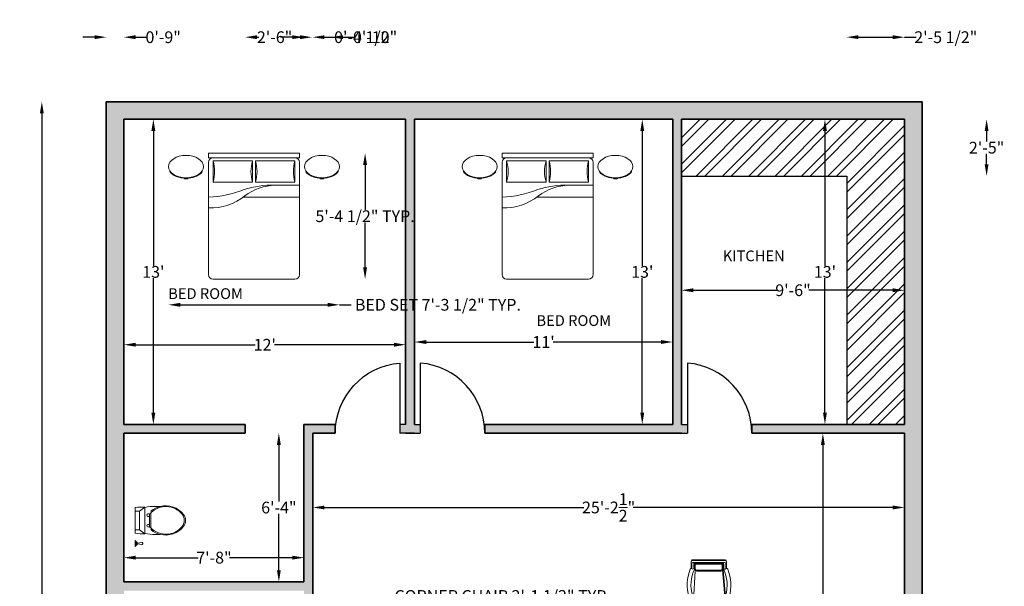
# Model space of a CAD drawing. Units: inches. Extents: x 2490 to 2996, y 1528 to 2269.
# Tile 4 of 4: x 2490 to 2993, y 1979 to 2269. Entities that reach past the tile are written whole.
import ezdxf

# ---------------------------------------------------------------- set-up
doc = ezdxf.new("R2010")
doc.units = ezdxf.units.IN
for name, color, linetype, lineweight in [('A-ANNO-DIMS', 2, 'Continuous', 18), ('A-DOOR', 4, 'Continuous', 25), ('A-FLOR-CASE', 7, 'Continuous', 25), ('A-FURN', 8, 'Continuous', 18), ('A-WALL', 7, 'Continuous', 35)]:
    doc.layers.add(name, color=color, linetype=linetype, lineweight=lineweight)
for name, color, linetype, lineweight, true_color in [('A-AREA-IDEN', 244, 'Continuous', 25, 0x991b1e), ('A-FLOR-CASE-PATT', 85, 'Continuous', 13, 0x58ba48), ('A-FLOR-FIXT', 244, 'Continuous', 18, 0x991b1e), ('A-WALL-PATT', 85, 'Continuous', 13, 0x58ba48)]:
    doc.layers.add(name, color=color, linetype=linetype, lineweight=lineweight, true_color=true_color)
doc.styles.get("Standard").update_dxf_attribs({"font": 'arial.ttf'})
doc.dimstyles.get("Standard").update_dxf_attribs({"dimtxt": 6, "dimasz": 6, "dimexe": 0.18, "dimexo": 0.0625, "dimgap": 0.09, "dimtad": 0, "dimtih": 1, "dimtoh": 1, "dimdec": 4, "dimzin": 0, "dimdsep": 46, "dimlunit": 4, "dimtxsty": 'Standard', "dimcen": 0.09, "dimse1": 1, "dimse2": 1, "dimadec": 0, "dimazin": 0, "dimtfac": 1, "dimtdec": 4, "dimtofl": 0, "dimtmove": 0, "dimatfit": 3, "dimfxl": 1, "dimtolj": 1, "dimtzin": 0, "dimarcsym": 0})

# ---------------------------------------------------------------- blocks, each defined once
blk = doc.blocks.new('*D7')
at = {"layer": 'A-ANNO-DIMS', "color": 0, "lineweight": -2, "transparency": 16777216}
for p, q in [((2549.28, 2102.88), (2610.38, 2102.88)), ((2681.28, 2102.88), (2620.18, 2102.88))]:
    blk.add_line(p, q, dxfattribs=at)
at = {"layer": 'A-ANNO-DIMS', "color": 0, "transparency": 16777216}
for points in [[(2549.28, 2103.88), (2549.28, 2101.88), (2543.28, 2102.88)], [(2681.28, 2103.88), (2681.28, 2101.88), (2687.28, 2102.88)]]:
    blk.add_solid(points, dxfattribs=at)
at = {"layer": 'Defpoints', "color": 0, "transparency": 16777216}
for p in [(2543.28, 2218.13), (2687.28, 2218.13), (2687.28, 2102.88)]:
    blk.add_point(p, dxfattribs=at)
at = {"layer": 'A-ANNO-DIMS', "color": 0, "transparency": 16777216, "insert": (2615.28, 2102.88), "char_height": 6, "attachment_point": 5}
blk.add_mtext("\\A1;12'", dxfattribs=at)
blk = doc.blocks.new('*D8')
at = {"layer": 'A-ANNO-DIMS', "color": 0, "lineweight": -2, "transparency": 16777216}
for p, q in [((2558.32, 2212.13), (2558.32, 2143.29)), ((2558.32, 2068.13), (2558.32, 2136.98))]:
    blk.add_line(p, q, dxfattribs=at)
at = {"layer": 'A-ANNO-DIMS', "color": 0, "transparency": 16777216}
for points in [[(2557.32, 2212.13), (2559.32, 2212.13), (2558.32, 2218.13)], [(2557.32, 2068.13), (2559.32, 2068.13), (2558.32, 2062.13)]]:
    blk.add_solid(points, dxfattribs=at)
at = {"layer": 'Defpoints', "color": 0, "transparency": 16777216}
for p in [(2687.28, 2218.13), (2558.32, 2062.13), (2687.28, 2062.13)]:
    blk.add_point(p, dxfattribs=at)
at = {"layer": 'A-ANNO-DIMS', "color": 0, "transparency": 16777216, "insert": (2558.32, 2140.13), "char_height": 6, "attachment_point": 5}
blk.add_mtext("\\A1;13'", dxfattribs=at)
blk = doc.blocks.new('*D9')
at = {"layer": 'A-ANNO-DIMS', "color": 0, "lineweight": -2, "transparency": 16777216}
for p, q in [((2808.24, 2212.13), (2808.24, 2143.29)), ((2808.24, 2068.13), (2808.24, 2136.98))]:
    blk.add_line(p, q, dxfattribs=at)
at = {"layer": 'A-ANNO-DIMS', "color": 0, "transparency": 16777216}
for points in [[(2807.24, 2212.13), (2809.24, 2212.13), (2808.24, 2218.13)], [(2807.24, 2068.13), (2809.24, 2068.13), (2808.24, 2062.13)]]:
    blk.add_solid(points, dxfattribs=at)
at = {"layer": 'Defpoints', "color": 0, "transparency": 16777216}
for p in [(2691.78, 2218.13), (2691.78, 2062.13), (2808.24, 2062.13)]:
    blk.add_point(p, dxfattribs=at)
at = {"layer": 'A-ANNO-DIMS', "color": 0, "transparency": 16777216, "insert": (2808.24, 2140.13), "char_height": 6, "attachment_point": 5}
blk.add_mtext("\\A1;13'", dxfattribs=at)
blk = doc.blocks.new('*D10')
at = {"layer": 'A-ANNO-DIMS', "color": 0, "lineweight": -2, "transparency": 16777216}
for p, q in [((2697.78, 2104.27), (2752.88, 2104.27)), ((2817.78, 2104.27), (2762.68, 2104.27))]:
    blk.add_line(p, q, dxfattribs=at)
at = {"layer": 'A-ANNO-DIMS', "color": 0, "transparency": 16777216}
for points in [[(2697.78, 2105.27), (2697.78, 2103.27), (2691.78, 2104.27)], [(2817.78, 2105.27), (2817.78, 2103.27), (2823.78, 2104.27)]]:
    blk.add_solid(points, dxfattribs=at)
at = {"layer": 'Defpoints', "color": 0, "transparency": 16777216}
for p in [(2691.78, 2218.13), (2823.78, 2218.13), (2823.78, 2104.27)]:
    blk.add_point(p, dxfattribs=at)
at = {"layer": 'A-ANNO-DIMS', "color": 0, "transparency": 16777216, "insert": (2757.78, 2104.27), "char_height": 6, "attachment_point": 5}
blk.add_mtext("\\A1;11'", dxfattribs=at)
blk = doc.blocks.new('*D11')
at = {"layer": 'A-ANNO-DIMS', "color": 0, "lineweight": -2, "transparency": 16777216}
for p, q in [((2834.28, 2130.74), (2877.21, 2130.74)), ((2936.28, 2130.74), (2893.34, 2130.74))]:
    blk.add_line(p, q, dxfattribs=at)
at = {"layer": 'A-ANNO-DIMS', "color": 0, "transparency": 16777216}
for points in [[(2834.28, 2131.74), (2834.28, 2129.74), (2828.28, 2130.74)], [(2936.28, 2131.74), (2936.28, 2129.74), (2942.28, 2130.74)]]:
    blk.add_solid(points, dxfattribs=at)
at = {"layer": 'Defpoints', "color": 0, "transparency": 16777216}
for p in [(2828.28, 2218.13), (2942.28, 2218.13), (2942.28, 2130.74)]:
    blk.add_point(p, dxfattribs=at)
at = {"layer": 'A-ANNO-DIMS', "color": 0, "transparency": 16777216, "insert": (2885.28, 2130.74), "char_height": 6, "attachment_point": 5}
blk.add_mtext('\\A1;9\'-6"', dxfattribs=at)
blk = doc.blocks.new('*D12')
at = {"layer": 'A-ANNO-DIMS', "color": 0, "lineweight": -2, "transparency": 16777216}
for p, q in [((2901.61, 2212.13), (2901.61, 2143.29)), ((2901.61, 2068.13), (2901.61, 2136.98))]:
    blk.add_line(p, q, dxfattribs=at)
at = {"layer": 'A-ANNO-DIMS', "color": 0, "transparency": 16777216}
for points in [[(2900.61, 2212.13), (2902.61, 2212.13), (2901.61, 2218.13)], [(2900.61, 2068.13), (2902.61, 2068.13), (2901.61, 2062.13)]]:
    blk.add_solid(points, dxfattribs=at)
at = {"layer": 'Defpoints', "color": 0, "transparency": 16777216}
for p in [(2828.28, 2218.13), (2828.28, 2062.13), (2901.61, 2062.13)]:
    blk.add_point(p, dxfattribs=at)
at = {"layer": 'A-ANNO-DIMS', "color": 0, "transparency": 16777216, "insert": (2901.61, 2140.13), "char_height": 6, "attachment_point": 5}
blk.add_mtext("\\A1;13'", dxfattribs=at)
blk = doc.blocks.new('*D13')
at = {"layer": 'A-ANNO-DIMS', "color": 0, "lineweight": -2, "transparency": 16777216}
for p, q in [((2900.56, 2051.63), (2900.56, 1910.79)), ((2900.56, 1763.63), (2900.56, 1904.48))]:
    blk.add_line(p, q, dxfattribs=at)
at = {"layer": 'A-ANNO-DIMS', "color": 0, "transparency": 16777216}
for points in [[(2899.56, 2051.63), (2901.56, 2051.63), (2900.56, 2057.63)], [(2899.56, 1763.63), (2901.56, 1763.63), (2900.56, 1757.63)]]:
    blk.add_solid(points, dxfattribs=at)
at = {"layer": 'Defpoints', "color": 0, "transparency": 16777216}
for p in [(2942.28, 2057.63), (2900.56, 1757.63), (2942.28, 1757.63)]:
    blk.add_point(p, dxfattribs=at)
at = {"layer": 'A-ANNO-DIMS', "color": 0, "transparency": 16777216, "insert": (2900.56, 1907.63), "char_height": 6, "attachment_point": 5}
blk.add_mtext("\\A1;25'", dxfattribs=at)
blk = doc.blocks.new('*D14')
at = {"layer": 'A-ANNO-DIMS', "color": 0, "lineweight": -2, "transparency": 16777216}
for p, q in [((2622.47, 2051.63), (2622.47, 2022.79)), ((2622.47, 1987.63), (2622.47, 2016.48))]:
    blk.add_line(p, q, dxfattribs=at)
at = {"layer": 'A-ANNO-DIMS', "color": 0, "transparency": 16777216}
for points in [[(2621.47, 2051.63), (2623.47, 2051.63), (2622.47, 2057.63)], [(2621.47, 1987.63), (2623.47, 1987.63), (2622.47, 1981.63)]]:
    blk.add_solid(points, dxfattribs=at)
at = {"layer": 'Defpoints', "color": 0, "transparency": 16777216}
for p in [(2543.28, 2057.63), (2543.28, 1981.63), (2622.47, 1981.63)]:
    blk.add_point(p, dxfattribs=at)
at = {"layer": 'A-ANNO-DIMS', "color": 0, "transparency": 16777216, "insert": (2622.47, 2019.63), "char_height": 6, "attachment_point": 5}
blk.add_mtext('\\A1;6\'-4"', dxfattribs=at)
blk = doc.blocks.new('*D15')
at = {"layer": 'A-ANNO-DIMS', "color": 0, "lineweight": -2, "transparency": 16777216}
for p, q in [((2549.28, 1994.02), (2581.24, 1994.02)), ((2629.28, 1994.02), (2597.32, 1994.02))]:
    blk.add_line(p, q, dxfattribs=at)
at = {"layer": 'A-ANNO-DIMS', "color": 0, "transparency": 16777216}
for points in [[(2549.28, 1995.02), (2549.28, 1993.02), (2543.28, 1994.02)], [(2629.28, 1995.02), (2629.28, 1993.02), (2635.28, 1994.02)]]:
    blk.add_solid(points, dxfattribs=at)
at = {"layer": 'Defpoints', "color": 0, "transparency": 16777216}
for p in [(2635.28, 1994.02), (2543.28, 1981.63), (2635.28, 1981.63)]:
    blk.add_point(p, dxfattribs=at)
at = {"layer": 'A-ANNO-DIMS', "color": 0, "transparency": 16777216, "insert": (2589.28, 1994.02), "char_height": 6, "attachment_point": 5}
blk.add_mtext('\\A1;7\'-8"', dxfattribs=at)
blk = doc.blocks.new('*D22')
at = {"layer": 'A-ANNO-DIMS', "color": 0, "lineweight": -2, "transparency": 16777216}
for p, q in [((2645.78, 2019.69), (2778.39, 2019.69)), ((2936.28, 2019.69), (2803.66, 2019.69))]:
    blk.add_line(p, q, dxfattribs=at)
at = {"layer": 'A-ANNO-DIMS', "color": 0, "transparency": 16777216}
for points in [[(2645.78, 2020.69), (2645.78, 2018.69), (2639.78, 2019.69)], [(2936.28, 2020.69), (2936.28, 2018.69), (2942.28, 2019.69)]]:
    blk.add_solid(points, dxfattribs=at)
at = {"layer": 'Defpoints', "color": 0, "transparency": 16777216}
for p in [(2639.78, 2032.5), (2942.28, 2032.5), (2942.28, 2019.69)]:
    blk.add_point(p, dxfattribs=at)
at = {"layer": 'A-ANNO-DIMS', "color": 0, "transparency": 16777216, "insert": (2791.03, 2019.69), "char_height": 6, "attachment_point": 5}
blk.add_mtext('\\A1;25\'-2{\\H1x;\\S1/2;}"', dxfattribs=at)
blk = doc.blocks.new('BED-WITH-NIGHTSTANDS')
for p, q in [((20.41, 64.37), (66.94, 64.37)), ((20.41, 62.04), (20.41, 64.37)), ((20.41, 62.04), (66.94, 62.04)), ((22.74, 60.49), (22.74, 49.63)), ((42.9, 60.49), (22.74, 60.49)), ((42.9, 49.63), (42.9, 60.49)), ((64.61, 60.49), (44.45, 60.49)), ((44.45, 60.49), (44.45, 49.63)), ((64.61, 49.63), (64.61, 60.49)), ((66.94, 62.04), (66.94, 64.37)), ((20.41, 2.33), (20.41, 59.72)), ((66.94, 59.72), (66.94, 2.33)), ((0.95, 54.97), (0.72, 54.79)), ((16.97, 54.97), (17.2, 54.79)), ((70.38, 54.97), (70.15, 54.79)), ((86.4, 54.97), (86.63, 54.79)), ((22.74, 49.63), (42.9, 49.63)), ((44.45, 49.63), (64.61, 49.63)), ((54.15, 48.08), (66.94, 48.08)), ((38.25, 41.88), (66.94, 41.88)), ((64.61, 0), (22.74, 0))]:
    blk.add_line(p, q)
for points in [[(9.82, 51.55), (9.82, 51.29), (8.1, 51.29), (8.1, 51.56)], [(77.53, 51.55), (77.53, 51.29), (79.25, 51.29), (79.25, 51.56)]]:
    blk.add_lwpolyline(points)
for centre, radius, start, end in [((22.74, 59.72), 2.33, 90, 180), ((4.12, 55.06), 19.39, 343.7398, 16.2602), ((61.51, 55.06), 19.39, 163.7398, 196.2602), ((25.84, 55.06), 19.39, 343.7398, 16.2602), ((83.23, 55.06), 19.39, 163.7398, 196.2602), ((64.61, 59.72), 2.33, 0, 90), ((17.8, 98.89), 57.07, 272.616, 291.4069), ((53.52, -0.58), 48.67, 89.2582, 107.8034), ((55.8, 19.6), 28.51, 92.5398, 126.0403), ((21.57, 63.79), 27.41, 267.5673, 309.5461), ((22.74, 2.33), 2.33, 180, 270), ((64.61, 2.33), 2.33, 270, 0)]:
    blk.add_arc(centre, radius, start, end)
blk.add_ellipse((8.96, 57.54), major_axis=(-8.96, 0), ratio=0.638095)
at = {"extrusion": (0, 0, -1)}
blk.add_ellipse((78.39, 57.54), major_axis=(8.96, 0), ratio=0.638095, dxfattribs=at)
for points in [[(0.72, 54.79), (0.84, 54.64), (0.96, 54.5), (3, 52.37), (6.73, 51.27), (13.16, 51.84), (15.82, 53.08), (17.2, 54.8)], [(86.63, 54.79), (86.51, 54.64), (86.39, 54.5), (84.35, 52.37), (80.63, 51.27), (74.19, 51.84), (71.53, 53.08), (70.15, 54.8)]]:
    blk.add_open_spline(points, degree=3, knots=[0.464624, 0.464624, 0.464624, 0.464624, 0.54806, 0.54806, 1.710779, 1.710779, 2.676847, 2.676847, 2.676847, 2.676847])
blk = doc.blocks.new('WC-PLAN')
for p, q in [((9.57, 17.88), (9.93, 18.54)), ((9.93, 18.54), (9.93, 19.26)), ((11.22, 18.54), (9.93, 18.54)), ((11.22, 19.26), (11.22, 18.54)), ((13.29, 18.54), (11.22, 18.54)), ((13.29, 18.54), (15.36, 18.54)), ((15.36, 19.26), (15.36, 18.54)), ((15.36, 18.54), (16.65, 18.54)), ((16.65, 18.54), (16.65, 19.26)), ((17.01, 17.88), (16.65, 18.54))]:
    blk.add_line(p, q)
for points in [[(2.96, 25.75), (0, 25.75)], [(2.78, 25.55), (0.18, 25.55)], [(2.16, 25.2), (0.8, 25.2)], [(0.8, 25.2), (0.8, 24.77), (1.28, 24.77)], [(1.15, 25.2), (1.15, 24.77)], [(1.71, 24.77), (2.14, 24.77), (2.16, 25.2)], [(1.84, 25.2), (1.84, 24.77)], [(6.49, 20.79), (8.51, 23.63), (8.51, 25.75)], [(19.81, 25.75), (6.76, 25.75)], [(20.09, 20.79), (18.06, 23.63), (18.06, 25.75)], [(1.28, 24.77), (1.71, 24.77)], [(6.61, 20.79), (13.29, 20.79)], [(8.51, 23.63), (13.29, 23.63)], [(18.06, 23.63), (13.29, 23.63)], [(19.96, 20.79), (13.29, 20.79)]]:
    blk.add_lwpolyline(points)
for points in [[(0.8, 25.2, -0.158381), (0, 25.75, 2.932383)], [(2.16, 25.2, 0.158381), (2.96, 25.75, -2.932383)], [(6.76, 25.75, 0.056711), (6.49, 20.79), (6.61, 20.79)], [(19.81, 25.75, -0.056711), (20.09, 20.79), (19.96, 20.79)], [(1.28, 24.75), (1.02, 22.39, 0.482607), (1.52, 21.9, -0.547905)], [(1.71, 24.75), (1.97, 22.39, -0.482607), (1.47, 21.9, 0.547905)], [(6.61, 20.78, 0.052121), (6.14, 15.38), (6.14, 13.01, 0.14456)], [(19.96, 20.78, -0.052121), (20.43, 15.38), (20.43, 13.01, -0.14456)], [(8.4, 17.61, 0.11024), (6.14, 13.01, 0.16845)], [(9.29, 17.61, 0.434217), (9.93, 1.97, 0.182634), (13.29, 0.75, 2.693815)], [(9.29, 17.61), (8.4, 17.61, 0.416606)], [(9.57, 17.88, 0.008985), (9.29, 17.61, 0.182634)], [(13.29, 17.88), (9.57, 17.88, 0.008985)], [(13.29, 17.88), (17.01, 17.88, -0.444938)], [(17.28, 17.61, -0.434217), (16.65, 1.97, -0.182634), (13.29, 0.75, -2.693815)], [(17.01, 17.88, -0.008985), (17.28, 17.61, -0.182634)], [(17.28, 17.61), (18.18, 17.61, -0.416606)], [(18.18, 17.61, -0.11024), (20.43, 13.01, -0.16845)], [(6.14, 13.01, 0.292914), (10.29, 1.04, 0.16845), (13.29, 0, 2.883082)], [(20.43, 13.01, -0.292914), (16.29, 1.04, -0.16845), (13.29, 0, -2.883082)]]:
    blk.add_lwpolyline(points, format="xyb")
for centre in [(10.57, 19.26), (16, 19.26)]:
    blk.add_arc(centre, 0.645, 0, 180)
blk = doc.blocks.new('DOOR-SINGLE-36IN')
for p, q in [((0, 36), (0, 4.5)), ((3, 35.88), (3, 0)), ((0, 4.5), (3, 4.5)), ((0, 0), (3, 0))]:
    blk.add_line(p, q)
blk.add_arc((0, 0), 36, 0, 85.2198)
blk = doc.blocks.new('CHAIR-DINING-END')
for p, q in [((1.03, 21.58), (1.03, 21.58)), ((1.03, 21.55), (1.17, 19.23)), ((1.55, 21.51), (1.65, 19.45)), ((2.41, 21.51), (2.55, 19.09)), ((2.87, 21.51), (2.92, 20.8)), ((2.91, 20.75), (3.01, 18.96)), ((3.3, 20.77), (4.13, 5.77)), ((3.7, 21.58), (19.05, 21.58)), ((3.7, 21.19), (19.05, 21.19)), ((19.44, 20.76), (18.02, 5.06)), ((19.83, 20.72), (18.42, 5.06)), ((19.9, 21.5), (19.79, 20.22)), ((20.41, 21.51), (20.2, 19.36)), ((21.27, 21.51), (21.08, 19.36)), ((21.32, 21.58), (21.32, 21.58)), ((21.75, 21.51), (21.52, 18.92)), ((4.99, 5.74), (17.19, 5.74)), ((5.13, 5.35), (17.19, 5.35)), ((2.01, 4.43), (2.01, 0.99)), ((2.41, 4.39), (2.41, 4.34)), ((2.41, 4.34), (2.41, 1.98)), ((2.6, 0.4), (19.53, 0.4)), ((2.6, 0.01), (19.53, 0.01)), ((3, 1.39), (19.14, 1.39)), ((3.39, 4.34), (3.39, 2.17)), ((3.4, 4.35), (3.73, 4.35)), ((3.41, 4.4), (3.42, 4.34)), ((3.76, 4.35), (3.76, 2.23)), ((3.78, 1.78), (18.35, 1.78)), ((4.15, 4.37), (4.15, 2.23)), ((17.97, 2.23), (4.15, 2.23)), ((17.97, 1.84), (4.15, 1.84)), ((17.97, 4.43), (17.97, 2.23)), ((18.36, 4.46), (18.36, 4.43)), ((18.37, 4.43), (18.37, 2.23)), ((18.75, 2.17), (18.75, 4.34)), ((18.75, 4.28), (18.75, 4.28)), ((19.73, 1.98), (19.73, 4.34)), ((19.74, 4.34), (20.05, 4.34)), ((20.12, 0.99), (20.12, 4.34))]:
    blk.add_line(p, q)
for centre, radius, start, end in [((1.3, 21.52), 0.264, 1.2493, 181.2491), ((1.99, 21.5), 0.433, 0.0001, 179.9999), ((2.65, 21.5), 0.226, 1.4574, 181.4572), ((3.7, 20.79), 0.787, 90, 183.1605), ((3.7, 20.79), 0.394, 90, 183.1605), ((19.05, 20.79), 0.787, 354.8251, 90), ((19.05, 20.79), 0.394, 354.8251, 90), ((20.16, 21.51), 0.25, 1.1824, 181.1823), ((20.84, 21.51), 0.429, 0.0001, 179.9999), ((21.51, 21.51), 0.243, 0.0001, 179.9999), ((20.42, 12.86), 20.42, 162.689, 203.1795), ((1.8, 18.45), 1.01, 353.9479, 163.3079), ((20.42, 12.86), 18.46, 162.689, 206.4635), ((2, 12.86), 18.46, 333.5666, 17.311), ((20.64, 18.48), 0.982, 15.3669, 195.3668), ((2, 12.86), 20.42, 336.8205, 17.311), ((4.99, 4.56), 1.18, 90, 171.0504), ((5.13, 4.37), 0.984, 90, 180), ((17.19, 4.56), 1.18, 354.8251, 90), ((17.19, 4.56), 0.787, 354.8251, 90), ((2.37, 5.13), 0.787, 203.1795, 270), ((2.6, 0.99), 0.591, 180, 269.9996), ((2.62, 0.41), 0.405, 180.0001, 270), ((3, 1.98), 0.591, 180, 269.9996), ((2.92, 4.33), 0.481, 0.0001, 179.9999), ((3.78, 2.17), 0.394, 180, 269.9996), ((3.73, 4.54), 0.197, 270, 26.4635), ((4.15, 2.23), 0.394, 180, 270), ((17.97, 2.23), 0.394, 270, 0), ((2, 12.86), 18.46, 332.2307, 332.4303), ((18.35, 2.17), 0.394, 269.9996, 359.9993), ((18.7, 4.55), 0.197, 153.5666, 239.4109), ((18.76, 4.65), 0.315, 239.4109, 270), ((19.26, 4.33), 0.498, 0.0001, 179.9999), ((19.14, 1.98), 0.591, 269.9996, 359.9993), ((19.53, 0.99), 0.591, 269.9996, 359.9993), ((19.54, 0.41), 0.405, 270, 359.9979), ((20.05, 5.13), 0.787, 270, 336.8205)]:
    blk.add_arc(centre, radius, start, end)
blk = doc.blocks.new('*D30')
at = {"layer": 'A-ANNO-DIMS', "color": 0, "lineweight": -2, "transparency": 16777216}
for p, q in [((2572.09, 2123.3), (2647.44, 2123.3)), ((2653.44, 2123.3), (2659.44, 2123.3))]:
    blk.add_line(p, q, dxfattribs=at)
at = {"layer": 'A-ANNO-DIMS', "color": 0, "transparency": 16777216}
for points in [[(2572.09, 2124.3), (2572.09, 2122.3), (2566.09, 2123.3)], [(2647.44, 2124.3), (2647.44, 2122.3), (2653.44, 2123.3)]]:
    blk.add_solid(points, dxfattribs=at)
at = {"layer": 'Defpoints', "color": 0, "transparency": 16777216}
for p in [(2566.09, 2136.41), (2653.44, 2136.41), (2653.44, 2123.3)]:
    blk.add_point(p, dxfattribs=at)
at = {"layer": 'A-ANNO-DIMS', "color": 0, "transparency": 16777216, "insert": (2703.77, 2123.3), "char_height": 6, "attachment_point": 5}
blk.add_mtext('\\A1;BED SET 7\'-3 1/2" TYP.', dxfattribs=at)
blk = doc.blocks.new('*D31')
at = {"layer": 'A-ANNO-DIMS', "color": 0, "lineweight": -2, "transparency": 16777216}
for p, q in [((2666.54, 2194.78), (2666.54, 2171.78)), ((2666.54, 2142.41), (2666.54, 2165.4))]:
    blk.add_line(p, q, dxfattribs=at)
at = {"layer": 'A-ANNO-DIMS', "color": 0, "transparency": 16777216}
for points in [[(2665.54, 2194.78), (2667.54, 2194.78), (2666.54, 2200.78)], [(2665.54, 2142.41), (2667.54, 2142.41), (2666.54, 2136.41)]]:
    blk.add_solid(points, dxfattribs=at)
at = {"layer": 'Defpoints', "color": 0, "transparency": 16777216}
for p in [(2653.44, 2200.78), (2666.54, 2200.78), (2653.44, 2136.41)]:
    blk.add_point(p, dxfattribs=at)
at = {"layer": 'A-ANNO-DIMS', "color": 0, "transparency": 16777216, "insert": (2666.54, 2168.59), "char_height": 6, "attachment_point": 5}
blk.add_mtext('\\A1;5\'-4 1/2" TYP.', dxfattribs=at)
blk = doc.blocks.new('*D40')
at = {"layer": 'A-ANNO-DIMS', "color": 0, "lineweight": -2, "transparency": 16777216}
for p, q in [((2801.71, 1974.44), (2795.71, 1974.44)), ((2821.13, 1974.44), (2807.71, 1974.44))]:
    blk.add_line(p, q, dxfattribs=at)
at = {"layer": 'A-ANNO-DIMS', "color": 0, "transparency": 16777216}
for points in [[(2807.71, 1975.44), (2807.71, 1973.44), (2801.71, 1974.44)], [(2821.13, 1975.44), (2821.13, 1973.44), (2827.13, 1974.44)]]:
    blk.add_solid(points, dxfattribs=at)
at = {"layer": 'Defpoints', "color": 0, "transparency": 16777216}
for p in [(2801.71, 1974.44), (2801.71, 1970.63), (2827.13, 1970.63)]:
    blk.add_point(p, dxfattribs=at)
at = {"layer": 'A-ANNO-DIMS', "color": 0, "transparency": 16777216, "insert": (2736.85, 1974.44), "char_height": 6, "attachment_point": 5}
blk.add_mtext('\\A1;CORNER CHAIR 2\'-1 1/2" TYP.', dxfattribs=at)
blk = doc.blocks.new('*D47')
at = {"layer": 'A-ANNO-DIMS', "color": 0, "lineweight": -2, "transparency": 16777216}
for p, q in [((2501.3, 2221.13), (2501.3, 1901.79)), ((2501.3, 1576.13), (2501.3, 1895.48))]:
    blk.add_line(p, q, dxfattribs=at)
at = {"layer": 'A-ANNO-DIMS', "color": 0, "transparency": 16777216}
for points in [[(2500.3, 2221.13), (2502.3, 2221.13), (2501.3, 2227.13)], [(2500.3, 1576.13), (2502.3, 1576.13), (2501.3, 1570.13)]]:
    blk.add_solid(points, dxfattribs=at)
at = {"layer": 'Defpoints', "color": 0, "transparency": 16777216}
for p in [(2501.3, 2227.13), (2534.28, 2227.13), (2758.28, 1570.13)]:
    blk.add_point(p, dxfattribs=at)
at = {"layer": 'A-ANNO-DIMS', "color": 0, "transparency": 16777216, "insert": (2501.3, 1898.63), "char_height": 6, "attachment_point": 5}
blk.add_mtext('\\A1;54\'-9"', dxfattribs=at)
blk = doc.blocks.new('*D54')
at = {"layer": 'A-ANNO-DIMS', "color": 0, "lineweight": -2, "transparency": 16777216}
for p, q in [((2633.28, 2260.11), (2627.28, 2260.11)), ((2655.28, 2260.11), (2661.28, 2260.11))]:
    blk.add_line(p, q, dxfattribs=at)
at = {"layer": 'A-ANNO-DIMS', "color": 0, "transparency": 16777216}
for points in [[(2633.28, 2261.11), (2633.28, 2259.11), (2639.28, 2260.11)], [(2655.28, 2261.11), (2655.28, 2259.11), (2649.28, 2260.11)]]:
    blk.add_solid(points, dxfattribs=at)
at = {"layer": 'Defpoints', "color": 0, "transparency": 16777216}
for p in [(2649.28, 2260.11), (2639.28, 1822.63), (2649.28, 1822.63)]:
    blk.add_point(p, dxfattribs=at)
at = {"layer": 'A-ANNO-DIMS', "color": 0, "transparency": 16777216, "insert": (2671.67, 2260.11), "char_height": 6, "attachment_point": 5}
blk.add_mtext('\\A1;0\'-10"', dxfattribs=at)
blk = doc.blocks.new('*D55')
at = {"layer": 'A-ANNO-DIMS', "color": 0, "lineweight": -2, "transparency": 16777216}
for p, q in [((2528.28, 2260.11), (2522.28, 2260.11)), ((2549.28, 2260.11), (2555.28, 2260.11))]:
    blk.add_line(p, q, dxfattribs=at)
at = {"layer": 'A-ANNO-DIMS', "color": 0, "transparency": 16777216}
for points in [[(2528.28, 2261.11), (2528.28, 2259.11), (2534.28, 2260.11)], [(2549.28, 2261.11), (2549.28, 2259.11), (2543.28, 2260.11)]]:
    blk.add_solid(points, dxfattribs=at)
at = {"layer": 'Defpoints', "color": 0, "transparency": 16777216}
for p in [(2543.28, 2260.11), (2534.28, 2227.13), (2543.28, 2218.13)]:
    blk.add_point(p, dxfattribs=at)
at = {"layer": 'A-ANNO-DIMS', "color": 0, "transparency": 16777216, "insert": (2563.34, 2260.11), "char_height": 6, "attachment_point": 5}
blk.add_mtext('\\A1;0\'-9"', dxfattribs=at)
blk = doc.blocks.new('*D56')
at = {"layer": 'A-ANNO-DIMS', "color": 0, "lineweight": -2, "transparency": 16777216}
for p, q in [((2629.28, 2260.11), (2623.28, 2260.11)), ((2645.78, 2260.11), (2651.78, 2260.11))]:
    blk.add_line(p, q, dxfattribs=at)
at = {"layer": 'A-ANNO-DIMS', "color": 0, "transparency": 16777216}
for points in [[(2629.28, 2261.11), (2629.28, 2259.11), (2635.28, 2260.11)], [(2645.78, 2261.11), (2645.78, 2259.11), (2639.78, 2260.11)]]:
    blk.add_solid(points, dxfattribs=at)
at = {"layer": 'Defpoints', "color": 0, "transparency": 16777216}
for p in [(2639.78, 2260.11), (2635.28, 2062.13), (2639.78, 2057.63)]:
    blk.add_point(p, dxfattribs=at)
at = {"layer": 'A-ANNO-DIMS', "color": 0, "transparency": 16777216, "insert": (2666.83, 2260.11), "char_height": 6, "attachment_point": 5}
blk.add_mtext('\\A1;0\'-4 1/2"', dxfattribs=at)
blk = doc.blocks.new('*D57')
at = {"layer": 'A-ANNO-DIMS', "color": 0, "lineweight": -2, "transparency": 16777216}
for p, q in [((2611.28, 2260.11), (2612.16, 2260.11)), ((2629.28, 2260.11), (2628.39, 2260.11))]:
    blk.add_line(p, q, dxfattribs=at)
at = {"layer": 'A-ANNO-DIMS', "color": 0, "transparency": 16777216}
for points in [[(2611.28, 2261.11), (2611.28, 2259.11), (2605.28, 2260.11)], [(2629.28, 2261.11), (2629.28, 2259.11), (2635.28, 2260.11)]]:
    blk.add_solid(points, dxfattribs=at)
at = {"layer": 'Defpoints', "color": 0, "transparency": 16777216}
for p in [(2635.28, 2260.11), (2605.28, 2062.13), (2635.28, 2062.13)]:
    blk.add_point(p, dxfattribs=at)
at = {"layer": 'A-ANNO-DIMS', "color": 0, "transparency": 16777216, "insert": (2620.28, 2260.11), "char_height": 6, "attachment_point": 5}
blk.add_mtext('\\A1;2\'-6"', dxfattribs=at)
blk = doc.blocks.new('*D58')
at = {"layer": 'A-ANNO-DIMS', "color": 0, "lineweight": -2, "transparency": 16777216}
for p, q in [((2918.73, 2260.11), (2936.28, 2260.11)), ((2942.28, 2260.11), (2948.28, 2260.11))]:
    blk.add_line(p, q, dxfattribs=at)
at = {"layer": 'A-ANNO-DIMS', "color": 0, "transparency": 16777216}
for points in [[(2918.73, 2261.11), (2918.73, 2259.11), (2912.73, 2260.11)], [(2936.28, 2261.11), (2936.28, 2259.11), (2942.28, 2260.11)]]:
    blk.add_solid(points, dxfattribs=at)
at = {"layer": 'Defpoints', "color": 0, "transparency": 16777216}
for p in [(2942.28, 2260.11), (2942.28, 2218.13), (2912.73, 2189.12)]:
    blk.add_point(p, dxfattribs=at)
at = {"layer": 'A-ANNO-DIMS', "color": 0, "transparency": 16777216, "insert": (2963.38, 2260.11), "char_height": 6, "attachment_point": 5}
blk.add_mtext('\\A1;2\'-5 1/2"', dxfattribs=at)
blk = doc.blocks.new('*D59')
at = {"layer": 'A-ANNO-DIMS', "color": 0, "lineweight": -2, "transparency": 16777216}
for p, q in [((2984.25, 2212.13), (2984.25, 2206.78)), ((2984.25, 2195.12), (2984.25, 2200.47))]:
    blk.add_line(p, q, dxfattribs=at)
at = {"layer": 'A-ANNO-DIMS', "color": 0, "transparency": 16777216}
for points in [[(2983.25, 2212.13), (2985.25, 2212.13), (2984.25, 2218.13)], [(2983.25, 2195.12), (2985.25, 2195.12), (2984.25, 2189.12)]]:
    blk.add_solid(points, dxfattribs=at)
at = {"layer": 'Defpoints', "color": 0, "transparency": 16777216}
for p in [(2942.28, 2218.13), (2984.25, 2218.13), (2912.73, 2189.12)]:
    blk.add_point(p, dxfattribs=at)
at = {"layer": 'A-ANNO-DIMS', "color": 0, "transparency": 16777216, "insert": (2984.25, 2203.63), "char_height": 6, "attachment_point": 5}
blk.add_mtext('\\A1;2\'-5"', dxfattribs=at)

msp = doc.modelspace()

# ---------------------------------------------------------------- hatches: boundary and pattern name
at = {"layer": 'A-FLOR-CASE-PATT'}
h = msp.add_hatch(dxfattribs=at)
h.set_pattern_fill('ANSI32', color=256)
h.paths.add_polyline_path([(2942.27862, 2218.13248), (2828.27862, 2218.13248), (2828.27862, 2189.1223), (2912.72981, 2189.1223), (2912.72981, 2062.13248), (2942.27862, 2062.13248)])
at = {"layer": 'A-WALL-PATT'}
h = msp.add_hatch(color=256, dxfattribs=at)
h.dxf.hatch_style = 1
h.paths.add_polyline_path([(2951.27862, 2227.13248), (2534.27862, 2227.13248), (2534.27862, 1594.13248), (2543.27862, 1594.13248), (2543.27862, 1776.13248), (2543.27862, 1780.63248), (2543.27862, 1788.13248), (2639.77862, 1788.13248), (2722.27862, 1788.13248), (2722.27862, 1792.63248), (2639.77862, 1792.63248), (2543.27862, 1792.63248), (2543.27862, 1822.63248), (2543.27862, 1876.63248), (2639.77862, 1876.63248), (2651.27862, 1876.63248), (2651.27862, 1881.13248), (2639.77862, 1881.13248), (2639.77862, 1884.13248), (2635.27862, 1884.13248), (2635.27862, 1881.13248), (2603.77862, 1881.13248), (2543.27862, 1881.13248), (2543.27862, 1977.13248), (2635.27862, 1977.13248), (2635.27862, 1917.13248), (2639.77862, 1917.13248), (2639.77862, 2057.63248), (2651.27862, 2057.63248), (2651.27862, 2062.13248), (2635.27862, 2062.13248), (2635.27862, 2057.63248), (2635.27862, 1981.63248), (2543.27862, 1981.63248), (2543.27862, 2057.63248), (2605.27862, 2057.63248), (2605.27862, 2062.13248), (2543.27862, 2062.13248), (2543.27862, 2218.13248), (2687.27862, 2218.13248), (2687.27862, 2062.13248), (2684.27862, 2062.13248), (2684.27862, 2057.63248), (2687.27862, 2057.63248), (2691.77862, 2057.63248), (2694.77862, 2057.63248), (2694.77862, 2062.13248), (2691.77862, 2062.13248), (2691.77862, 2093.63248), (2691.77862, 2218.13248), (2823.77862, 2218.13248), (2823.77862, 2062.13248), (2727.77862, 2062.13248), (2727.77862, 2057.63248), (2828.27862, 2057.63248), (2831.27862, 2057.63248), (2831.27862, 2062.13248), (2828.27862, 2062.13248), (2828.27862, 2093.63248), (2828.27862, 2218.13248), (2942.27862, 2218.13248), (2942.27862, 2062.13248), (2864.27862, 2062.13248), (2864.27862, 2057.63248), (2942.27862, 2057.63248), (2942.27862, 1757.63248), (2834.77862, 1757.63248), (2834.77862, 1753.13248), (2942.27862, 1753.13248), (2942.27862, 1609.13248), (2798.77862, 1609.13248), (2798.77862, 1600.13248), (2951.27862, 1600.13248)])
h.paths.add_polyline_path([(2798.77862, 1753.13248), (2801.77862, 1753.13248), (2801.77862, 1757.63248), (2798.77862, 1757.63248), (2798.77862, 1780.63248), (2798.77862, 1792.63248), (2794.27862, 1792.63248), (2794.27862, 1788.13248), (2794.27862, 1776.13248), (2794.27862, 1757.63248), (2794.27862, 1594.13248), (2798.77862, 1594.13248)], flags=17)

# ---------------------------------------------------------------- linework, layer by layer
at = {"layer": 'A-FLOR-CASE'}
for p, q in [((2828.27862, 2189.1223), (2912.72981, 2189.1223)), ((2912.72981, 2189.1223), (2912.72981, 2062.13248))]:
    msp.add_line(p, q, dxfattribs=at)
at = {"layer": 'A-WALL'}
for p, q in [((2534.27862, 2227.13248), (2534.27862, 1594.13248)), ((2534.27862, 2227.13248), (2951.27862, 2227.13248)), ((2951.27862, 2227.13248), (2951.27862, 1600.13248)), ((2543.27862, 2218.13248), (2543.27862, 2062.13248)), ((2543.27862, 2218.13248), (2687.27862, 2218.13248)), ((2687.27862, 2218.13248), (2687.27862, 2062.13248)), ((2687.27862, 2218.13248), (2687.27862, 2062.13248)), ((2691.77862, 2218.13248), (2691.77862, 2062.13248)), ((2691.77862, 2218.13248), (2823.77862, 2218.13248)), ((2823.77862, 2218.13248), (2823.77862, 2062.13248)), ((2828.27862, 2218.13248), (2828.27862, 2062.13248)), ((2828.27862, 2218.13248), (2942.27862, 2218.13248)), ((2942.27862, 2218.13248), (2942.27862, 2062.13248)), ((2543.27862, 2062.13248), (2605.27862, 2062.13248)), ((2605.27862, 2062.13248), (2605.27862, 2057.63248)), ((2635.27862, 2057.63248), (2635.27862, 2062.13248)), ((2635.27862, 2062.13248), (2651.27862, 2062.13248)), ((2651.27862, 2057.63248), (2651.27862, 2062.13248)), ((2727.77862, 2062.13248), (2823.77862, 2062.13248)), ((2727.77862, 2057.63248), (2727.77862, 2062.13248)), ((2864.27862, 2057.63248), (2864.27862, 2062.13248)), ((2864.27862, 2062.13248), (2942.27862, 2062.13248)), ((2543.27862, 2057.63248), (2605.27862, 2057.63248)), ((2543.27862, 2057.63248), (2543.27862, 1981.63248)), ((2635.27862, 2057.63248), (2635.27862, 1981.63248)), ((2639.77862, 2057.63248), (2639.77862, 1917.13248)), ((2639.77862, 2057.63248), (2651.27862, 2057.63248)), ((2687.27862, 2057.63248), (2691.77862, 2057.63248)), ((2727.77862, 2057.63248), (2828.27862, 2057.63248)), ((2864.27862, 2057.63248), (2942.27862, 2057.63248)), ((2942.27862, 2057.63248), (2942.27862, 1757.63248)), ((2543.27862, 1981.63248), (2635.27862, 1981.63248))]:
    msp.add_line(p, q, dxfattribs=at)

# ---------------------------------------------------------------- block references
at = {"layer": 'A-DOOR', "extrusion": (0, 0, -1), "zscale": -1}
msp.add_blockref('DOOR-SINGLE-36IN', (-2687.27825, 2057.632), dxfattribs=at)
at = {"layer": 'A-DOOR'}
for p in [(2691.779, 2057.632), (2828.279, 2057.632)]:
    msp.add_blockref('DOOR-SINGLE-36IN', p, dxfattribs=at)
at = {"layer": 'A-FLOR-FIXT', "rotation": 90.00000000001143}
msp.add_blockref('WC-PLAN', (2574.83119, 1999.78175), dxfattribs=at)
at = {"layer": 'A-FURN'}
for p in [(2566.086, 2136.407), (2716.1414, 2136.407)]:
    msp.add_blockref('BED-WITH-NIGHTSTANDS', p, dxfattribs=at)
at = {"layer": 'A-FURN', "extrusion": (0, 0, -1), "zscale": -1, "rotation": 180}
msp.add_blockref('CHAIR-DINING-END', (-2831.151, 1992.91253), dxfattribs=at)

# ---------------------------------------------------------------- texts
at = {"layer": 'A-AREA-IDEN', "char_height": 5.501423, "attachment_point": 1}
for s, insert in [('KITCHEN', (2849.37079, 2151.06601)), ('BED ROOM ', (2565.90819, 2131.7586)), ('BED ROOM ', (2754.14173, 2117.99263))]:
    msp.add_mtext_dynamic_manual_height_columns(s, width=200.8472283, gutter_width=27.50711, heights=[0], dxfattribs=dict(at, insert=insert))

# ---------------------------------------------------------------- dimensions: what is measured, and where the dimension line sits
at = {"layer": 'A-ANNO-DIMS'}
for base, p1, p2, override, picture, middle in [((2639.77862, 2260.10748), (2635.27862, 2062.13248), (2639.77862, 2057.63248), {"dimdec": 1, "dimlfac": 1, "dimrnd": 0, "dimzin": 1, "dimdsep": 46, "dimlunit": 4, "dimfrac": 2}, '*D56', (2666.83384, 2260.10748)), ((2942.27862, 2260.10748), (2912.72981, 2189.1223), (2942.27862, 2218.13248), {"dimdec": 1, "dimlfac": 1, "dimrnd": 0, "dimzin": 1, "dimdsep": 46, "dimlunit": 4, "dimfrac": 2}, '*D58', (2963.385, 2260.10748)), ((2543.27862, 2260.10748), (2534.27862, 2227.13248), (2543.27862, 2218.13248), {"dimdec": 1, "dimlfac": 1, "dimrnd": 0, "dimzin": 1, "dimdsep": 46, "dimlunit": 4, "dimfrac": 2}, '*D55', (2563.34339, 2260.10748)), ((2635.27862, 2260.10748), (2605.27862, 2062.13248), (2635.27862, 2062.13248), {"dimdec": 1, "dimlfac": 1, "dimrnd": 0, "dimzin": 1, "dimdsep": 46, "dimlunit": 4, "dimfrac": 2}, '*D57', (2620.27862, 2260.10748)), ((2649.27862, 2260.10748), (2639.27862, 1822.63248), (2649.27862, 1822.63248), {"dimdec": 1, "dimlfac": 1, "dimrnd": 0, "dimzin": 1, "dimdsep": 46, "dimlunit": 4, "dimfrac": 2}, '*D54', (2671.67422, 2260.10748)), ((2687.27862, 2102.88147), (2543.27862, 2218.13248), (2687.27862, 2218.13248), {"dimclrd": 0, "dimclre": 0, "dimclrt": 0}, '*D7', (2615.27862, 2102.88147)), ((2823.77862, 2104.27425), (2691.77862, 2218.13248), (2823.77862, 2218.13248), {"dimclrd": 0, "dimclre": 0, "dimclrt": 0}, '*D10', (2757.77862, 2104.27425)), ((2942.27862, 2130.73711), (2828.27862, 2218.13248), (2942.27862, 2218.13248), {"dimclrd": 0, "dimclre": 0, "dimclrt": 0}, '*D11', (2885.27862, 2130.73711)), ((2942.27862, 2019.695), (2639.77862, 2032.50067), (2942.27862, 2032.50067), {"dimclrd": 0, "dimclre": 0, "dimclrt": 0}, '*D22', (2791.02862, 2019.695)), ((2635.27862, 1994.02237), (2543.27862, 1981.63248), (2635.27862, 1981.63248), {"dimclrd": 0, "dimclre": 0, "dimclrt": 0}, '*D15', (2589.27862, 1994.02237))]:
    dim = msp.add_linear_dim(base=base, p1=p1, p2=p2, dimstyle='Standard', override=override, dxfattribs=at)
    dim.commit()
    dim.dimension.update_dxf_attribs({"geometry": picture, "text_midpoint": middle})
for base, p1, p2, override, picture, middle in [((2501.30362, 2227.13248), (2758.27862, 1570.13248), (2534.27862, 2227.13248), {"dimdec": 1, "dimlfac": 1, "dimrnd": 0, "dimzin": 1, "dimdsep": 46, "dimlunit": 4, "dimfrac": 2}, '*D47', (2501.30362, 1898.63248)), ((2558.31856, 2062.13248), (2687.27862, 2218.13248), (2687.27862, 2062.13248), {"dimclrd": 0, "dimclre": 0, "dimclrt": 0}, '*D8', (2558.31856, 2140.13248)), ((2808.24005, 2062.13248), (2691.77862, 2218.13248), (2691.77862, 2062.13248), {"dimclrd": 0, "dimclre": 0, "dimclrt": 0}, '*D9', (2808.24005, 2140.13248)), ((2901.61221, 2062.13248), (2828.27862, 2218.13248), (2828.27862, 2062.13248), {"dimclrd": 0, "dimclre": 0, "dimclrt": 0}, '*D12', (2901.61221, 2140.13248)), ((2984.25362, 2218.13248), (2912.72981, 2189.1223), (2942.27862, 2218.13248), {"dimdec": 1, "dimlfac": 1, "dimrnd": 0, "dimzin": 1, "dimdsep": 46, "dimlunit": 4, "dimfrac": 2}, '*D59', (2984.25362, 2203.62739)), ((2622.46839, 1981.63248), (2543.27862, 2057.63248), (2543.27862, 1981.63248), {"dimclrd": 0, "dimclre": 0, "dimclrt": 0}, '*D14', (2622.46839, 2019.63248)), ((2900.55659, 1757.63248), (2942.27862, 2057.63248), (2942.27862, 1757.63248), {"dimclrd": 0, "dimclre": 0, "dimclrt": 0}, '*D13', (2900.55659, 1907.63248))]:
    dim = msp.add_linear_dim(base=base, p1=p1, p2=p2, angle=90, dimstyle='Standard', override=override, dxfattribs=at)
    dim.commit()
    dim.dimension.update_dxf_attribs({"geometry": picture, "text_midpoint": middle})
for base, p1, p2, angle, text, picture, middle in [((2666.53943, 2200.7762), (2653.43681, 2136.40677), (2653.43681, 2200.7762), 90, '<> TYP.', '*D31', (2666.53943, 2168.59148)), ((2801.71476, 1974.44006), (2827.13382, 1970.6272), (2801.71476, 1970.6272), 180, 'CORNER CHAIR <> TYP.', '*D40', (2736.85259, 1974.44006))]:
    dim = msp.add_linear_dim(base=base, p1=p1, p2=p2, angle=angle, text=text, dimstyle='Standard', override={"dimdec": 1, "dimlfac": 1, "dimrnd": 0, "dimzin": 1, "dimdsep": 46, "dimlunit": 4, "dimfrac": 2}, dxfattribs=at)
    dim.commit()
    dim.dimension.update_dxf_attribs({"geometry": picture, "text_midpoint": middle})
dim = msp.add_linear_dim(base=(2653.43681, 2123.30415), p1=(2566.08601, 2136.40677), p2=(2653.43681, 2136.40677), text='BED SET <> TYP.', dimstyle='Standard', override={"dimdec": 1, "dimlfac": 1, "dimrnd": 0, "dimzin": 1, "dimdsep": 46, "dimlunit": 4, "dimfrac": 2}, dxfattribs=at)
dim.commit()
dim.dimension.update_dxf_attribs({"geometry": '*D30', "text_midpoint": (2703.7676, 2123.30415)})

doc.saveas('drawing.dxf')
